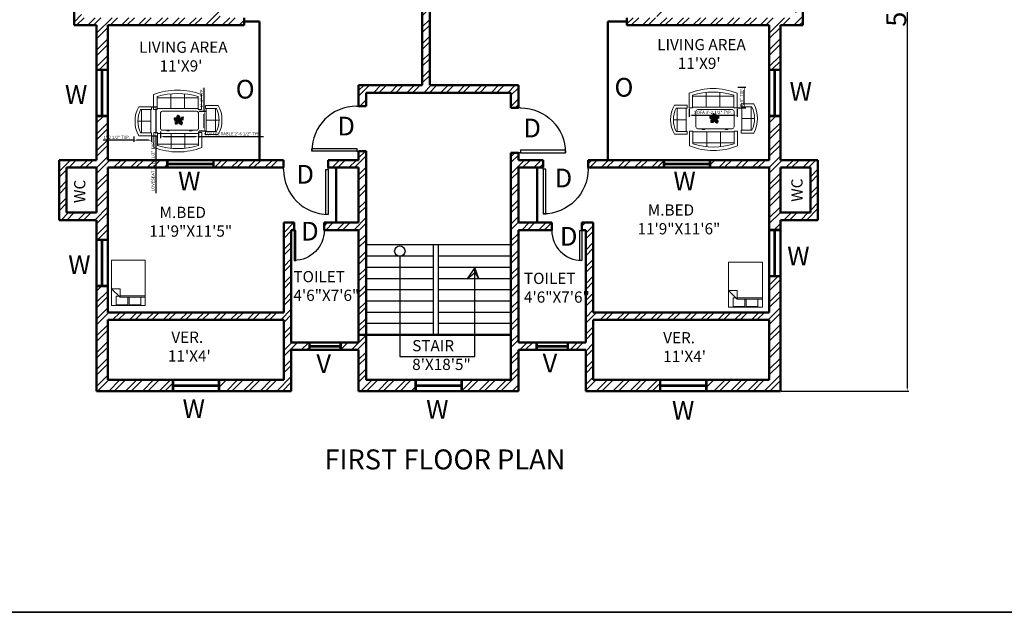
# Model space of a CAD drawing. Units: inches. Extents: x -31485 to -28799, y 18003 to 19130.
# Tile 8 of 15: x -30506 to -29717, y 18003 to 18478. Entities that reach past the tile are written whole.
import ezdxf

# ---------------------------------------------------------------- set-up
doc = ezdxf.new("R2010")
doc.units = ezdxf.units.IN
for name, color, linetype, lineweight in [('A-ANNO-DIMS', 2, 'Continuous', 18), ('A-ANNO-TEXT', 7, 'Continuous', 18), ('A-ANNO-TTLB', 7, 'Continuous', 35), ('A-AREA-IDEN', 7, 'Continuous', 18), ('A-DOOR', 3, 'Continuous', 25), ('A-FLOR-STRS', 3, 'Continuous', 25), ('A-FURN', 8, 'Continuous', 18), ('A-GLAZ', 4, 'Continuous', 25), ('A-WALL', 7, 'Continuous', 50), ('A-WALL-PATT', 8, 'Continuous', 13)]:
    doc.layers.add(name, color=color, linetype=linetype, lineweight=lineweight)
doc.styles.get("Standard").update_dxf_attribs({"font": 'arial.ttf'})
doc.dimstyles.new('ISO-25', dxfattribs={"dimtxt": 2.5, "dimasz": 2.5, "dimexe": 1.25, "dimexo": 0.625, "dimtad": 1, "dimdec": 0, "dimlunit": 3, "dimtxsty": 'Standard', "dimcen": 2.5, "dimadec": 0, "dimazin": 0, "dimtfac": 1, "dimtdec": 0, "dimtmove": 0, "dimatfit": 3, "dimfxl": 1, "dimarcsym": 0})

# ---------------------------------------------------------------- blocks, each defined once
blk = doc.blocks.new('*U8')
for p, q in [((0, 0), (0, -100)), ((750, 0), (750, -100))]:
    blk.add_line(p, q)
blk.add_lwpolyline([(0, 0), (0, 750), (43.75, 750), (43.75, 0)], close=True)
blk.add_arc((0, 0), 750, 0, 90)
blk = doc.blocks.new('Bed - Queen')
for p, q in [((0, -80.00003), (0, 0)), ((0, 0), (59.99999, 0)), ((59.99999, 0), (59.99999, -80.00003)), ((0, -14.4), (44.8, -14.4)), ((44.8, -16.8), (0, -16.8)), ((7.99999, -1.2), (28.79998, -1.2)), ((7.99999, -14.4), (7.99999, -1.2)), ((28.79998, -1.2), (28.79998, -14.4)), ((31.19999, -1.2), (51.99999, -1.2)), ((31.19999, -14.4), (31.19999, -1.2)), ((59.99999, -29.6), (44.8, -14.4)), ((44.8, -14.4), (44.8, -29.6)), ((51.99999, -16.4), (46.79936, -16.4)), ((51.99999, -1.2), (51.99999, -16.4)), ((44.8, -29.6), (59.99999, -29.6)), ((59.99999, -80.00003), (0, -80.00003))]:
    blk.add_line(p, q)
blk = doc.blocks.new('Desk - 30 x 60 in.')
for p, q in [((-26.999995, 0), (26.999995, 0)), ((-29.999995, -27), (-29.999995, -3)), ((29.999995, -3), (29.999995, -27)), ((26.999995, -30), (-26.999995, -30)), ((-20.000005, -30), (-20.000005, -31)), ((-16.000005, -31), (-16.000005, -30)), ((15.999995, -31), (15.999995, -30)), ((19.999995, -30), (19.999995, -31)), ((-20.000005, -31), (-16.000005, -31)), ((19.999995, -31), (15.999995, -31))]:
    blk.add_line(p, q)
for centre, start, end in [((-26.499995, -3.5), 98.1301, 171.8699), ((26.499995, -3.5), 8.130102, 81.8699), ((-26.499995, -26.5), 188.1301, 261.8699), ((26.499995, -26.5), 278.1301, 351.8699)]:
    blk.add_arc(centre, 3.535534, start, end)
blk = doc.blocks.new('Sofa - Roundback 7 ft.')
for p, q in [((-36.000027, -34), (-36.000027, -11.4696)), ((-35.999844, -13.3819), (35.9998, -13.3819)), ((-12.00002, -32.4421), (-12.00003, -6.5971)), ((11.99997, -32.4421), (11.99998, -6.5971)), ((35.99998, -34), (35.99998, -11.4696)), ((-36.000027, -32.4421), (35.99998, -32.4421))]:
    blk.add_line(p, q)
for points in [[(-36.000027, -34), (-42.000027, -34), (-42.000027, -8)], [(41.99998, -8), (41.99998, -34), (35.99998, -34)]]:
    blk.add_lwpolyline(points)
for centre, radius, start, end in [((0, -114.25), 114.25, 68.43141, 111.5686), ((-0.00001, -127.1968), 121.1968, 72.72033, 107.2797)]:
    blk.add_arc(centre, radius, start, end)
blk = doc.blocks.new('Sofa - Roundback Loveseat 5 ft.')
for p, q in [((-24, -33.99998), (-24, -11.46958)), ((-23.9998, -13.38178), (23.99986, -13.38178)), ((0, -32.44198), (0, -5.99998)), ((24.00004, -33.99998), (24.00004, -11.46958)), ((-24, -32.44198), (24.00004, -32.44198))]:
    blk.add_line(p, q)
for points in [[(-24, -33.99998), (-30, -33.99998), (-30, -7.99998)], [(30.00004, -7.99998), (30.00004, -33.99998), (24.00004, -33.99998)]]:
    blk.add_lwpolyline(points)
for centre, radius, start, end in [((0, -60.24998), 60.24998, 60.13715, 119.8628), ((0, -61.38438), 55.38444, 64.32083, 115.6792)]:
    blk.add_arc(centre, radius, start, end)
blk = doc.blocks.new('*U122')
for p, q in [((-1206.4492, 501.3198), (-1418.082, 465.9376)), ((-1031.621, 347.98), (-1399.667, 277.1902)), ((-800.1, 114.3), (-1333.5, 647.7)), ((-847.598, 159.2326), (-1326.0578, 135.636)), ((-1234.059, 536.7274), (-1252.4486, 737.2604)), ((-718.7946, 88.4682), (-1215.644, -147.447)), ((-1105.2302, 725.4494), (-1077.6458, 395.1732)), ((-976.4268, 666.4706), (-884.4026, 194.6402)), ((-543.9664, 76.6572), (-967.2066, -206.4512)), ((-902.8176, 713.6638), (-617.5756, 100.2538)), ((0, 0), (-800.1, 114.3)), ((-369.1382, 53.086), (-783.1836, 642.874)), ((-405.9428, 53.086), (-764.794, -241.8334)), ((-93.091, 489.5342), (-700.3796, 902.3858)), ((-129.8956, 713.6638), (-626.7704, 1032.1544)), ((-617.5756, 607.4918), (-74.7014, 347.98)), ((0, 0), (-571.5, -495.3)), ((-185.1152, 1008.5578), (-553.1612, 1185.4942)), ((-166.7002, 29.4894), (-543.9664, -206.4512)), ((-525.5514, 347.98), (-28.6766, 123.8504)), ((-221.9198, 1197.3052), (-433.5526, 1338.8594)), ((-258.7244, 1362.456), (-332.3336, 1421.4348)), ((0, 0), (-266.7, 1447.8)), ((-231.1146, 1315.2628), (-166.7002, 1421.4348)), ((-194.31, 1102.9442), (-65.4812, 1256.284)), ((-148.3106, 914.1968), (118.5418, 1220.9018)), ((-129.8956, 701.8528), (265.7602, 1185.4942)), ((-74.7014, 418.7444), (219.7608, 961.39)), ((-28.6766, 171.0436), (228.9556, 678.2816)), ((0, 0), (685.8, 228.6)), ((0, 0), (457.2, -571.5)), ((100.1268, 41.275), (284.1498, 619.2774)), ((164.5412, 41.275), (661.416, -218.2368)), ((256.5654, 88.4682), (449.7832, 666.4706)), ((284.1498, 88.4682), (781.0246, -147.447)), ((412.9786, 147.447), (587.8068, 796.2392)), ((458.978, 147.447), (891.4384, -88.4682)), ((560.197, 182.8292), (698.2206, 819.8358)), ((615.4166, 194.6402), (1185.8752, 41.275)), ((685.8, 228.6), (1219.2, 914.4)), ((689.0258, 230.0224), (790.2448, 914.1968)), ((753.4148, 312.5978), (1222.6798, 159.2326)), ((808.6344, 784.4282), (827.0494, 418.7444)), ((845.439, 418.7444), (1241.0948, 277.1902)), ((891.4384, 831.6214), (946.658, 572.1096)), ((919.0482, 501.3198), (1222.6798, 454.152)), ((983.4626, 867.0036), (1066.2666, 725.4494)), ((1029.462, 654.685), (1241.0948, 631.0884)), ((1112.2914, 760.8316), (1296.3144, 784.4282)), ((1121.4862, 925.9824), (1149.0706, 831.6214)), ((-442.7474, -383.3876), (-1086.8406, -477.7486)), ((-718.7946, -737.2604), (-1086.8406, -796.2392)), ((-617.5756, -548.5384), (-1077.6458, -560.324)), ((-783.1836, -867.029), (-1077.6458, -902.4112)), ((-875.2078, -1008.5832), (-1040.8412, -1079.3476)), ((-681.9646, -666.496), (-1022.4262, -654.685)), ((-571.5, -495.3), (-952.5, -1143)), ((-829.2084, -937.7934), (-810.7934, -1126.5408)), ((-387.5278, -324.4088), (-764.794, -324.4088)), ((-737.1842, -784.4536), (-709.5744, -1114.7298)), ((-635.9652, -607.5172), (-580.771, -1150.1374)), ((-525.5514, -465.963), (-451.9422, -1126.5408)), ((-166.7002, -147.447), (-507.1618, -253.619)), ((-433.5526, -383.3876), (-323.1134, -1020.3688)), ((-341.5284, -289.0012), (-221.9198, -831.6214)), ((-240.3094, -218.2368), (-157.5054, -595.7062)), ((-120.7008, -88.4682), (-93.091, -371.5766)), ((63.3222, -76.6826), (-37.8714, -513.1308)), ((44.9326, -64.897), (615.4166, -241.8334)), ((127.7366, -159.258), (54.1274, -654.685)), ((228.9556, -289.0012), (90.932, -914.1968)), ((357.759, -430.5554), (164.5412, -1020.3688)), ((192.151, -230.0224), (817.8292, -371.5766)), ((458.978, -572.1096), (210.5406, -1161.923)), ((311.7596, -383.3876), (937.4378, -477.7486)), ((514.1976, -772.6426), (403.7838, -1138.3264)), ((412.9786, -501.3452), (919.0482, -583.9206)), ((457.2, -571.5), (685.8, -1333.5)), ((468.1982, -572.1096), (1029.462, -737.2604)), ((486.5878, -642.8994), (983.4626, -843.4324)), ((578.612, -961.39), (495.7826, -1232.7128)), ((541.8074, -831.6214), (992.6574, -1032.1544)), ((578.612, -973.1756), (873.0488, -1138.3264)), ((624.6114, -1161.923), (587.8068, -1291.6916)), ((624.6114, -1102.9442), (781.0246, -1209.1162)), ((679.8056, -1268.095), (716.6102, -1291.6916))]:
    blk.add_line(p, q)
blk = doc.blocks.new('*D189')
at = {"layer": 'A-ANNO-DIMS', "color": 0, "lineweight": -2, "transparency": 16777216}
for p, q in [((-29895.58, 18824.12), (-29793.36, 18824.12)), ((-29794.61, 18821.62), (-29794.61, 18182.62)), ((-29895.58, 18180.12), (-29793.36, 18180.12))]:
    blk.add_line(p, q, dxfattribs=at)
at = {"layer": 'A-ANNO-DIMS', "color": 0, "transparency": 16777216}
for points in [[(-29795.03, 18821.62), (-29794.19, 18821.62), (-29794.61, 18824.12)], [(-29795.03, 18182.62), (-29794.19, 18182.62), (-29794.61, 18180.12)]]:
    blk.add_solid(points, dxfattribs=at)
at = {"layer": 'Defpoints', "color": 0, "transparency": 16777216}
for p in [(-29896.21, 18824.12), (-29896.21, 18180.12), (-29794.61, 18180.12)]:
    blk.add_point(p, dxfattribs=at)
at = {"layer": 'A-ANNO-DIMS', "color": 0, "transparency": 16777216, "insert": (-29803.41, 18502.12), "char_height": 2.5, "attachment_point": 5, "rotation": 90}
blk.add_mtext('{\\H6.4x;53\'-8"}', dxfattribs=at)
blk = doc.blocks.new('WIN-900-W9')
for p, q in [((-29982.21, 18824.12), (-29982.21, 18815.12)), ((-29981.21, 18824.12), (-29981.21, 18815.12)), ((-29981.21, 18820.12), (-29945.21, 18820.12)), ((-29981.21, 18819.62), (-29945.21, 18819.62)), ((-29981.21, 18819.12), (-29945.21, 18819.12)), ((-29945.21, 18824.12), (-29945.21, 18815.12)), ((-29944.21, 18824.12), (-29944.21, 18815.12))]:
    blk.add_line(p, q)
blk = doc.blocks.new('WIN-900-W6')
for p, q in [((-30183.21, 18720.12), (-30177.21, 18720.12)), ((-30183.21, 18719.12), (-30177.21, 18719.12)), ((-30180.71, 18683.12), (-30180.71, 18719.12)), ((-30180.21, 18683.12), (-30180.21, 18719.12)), ((-30179.71, 18683.12), (-30179.71, 18719.12)), ((-30183.21, 18683.12), (-30177.21, 18683.12)), ((-30183.21, 18682.12), (-30177.21, 18682.12))]:
    blk.add_line(p, q)
blk = doc.blocks.new('VENT-600-W6')
for p, q in [((-29884.21, 18519.12), (-29878.21, 18519.12)), ((-29884.21, 18518.12), (-29878.21, 18518.12)), ((-29881.71, 18494.12), (-29881.71, 18518.12)), ((-29881.21, 18494.12), (-29881.21, 18518.12)), ((-29880.71, 18494.12), (-29880.71, 18518.12)), ((-29884.21, 18494.12), (-29878.21, 18494.12)), ((-29884.21, 18493.12), (-29878.21, 18493.12))]:
    blk.add_line(p, q)
blk = doc.blocks.new('*D224')
at = {"layer": 'A-ANNO-DIMS', "color": 0, "lineweight": -2, "transparency": 16777216}
for p, q in [((-30399.59, 18407.94), (-30395.47, 18407.94)), ((-30396.72, 18405.44), (-30396.72, 18387.1)), ((-30399.59, 18384.6), (-30395.47, 18384.6)), ((-30396.72, 18384.6), (-30396.72, 18338.55))]:
    blk.add_line(p, q, dxfattribs=at)
at = {"layer": 'A-ANNO-DIMS', "color": 0, "transparency": 16777216}
for points in [[(-30397.13, 18405.44), (-30396.3, 18405.44), (-30396.72, 18407.94)], [(-30397.13, 18387.1), (-30396.3, 18387.1), (-30396.72, 18384.6)]]:
    blk.add_solid(points, dxfattribs=at)
at = {"layer": 'Defpoints', "color": 0, "transparency": 16777216}
for p in [(-30400.22, 18407.94), (-30400.22, 18384.6), (-30396.72, 18384.6)]:
    blk.add_point(p, dxfattribs=at)
at = {"layer": 'A-ANNO-DIMS', "color": 0, "transparency": 16777216, "insert": (-30398.63, 18360.33), "char_height": 2.5, "attachment_point": 5, "rotation": 90}
blk.add_mtext('LOVESEAT 1\'-11 1/2" TYP.', dxfattribs=at)
blk = doc.blocks.new('*D225')
at = {"layer": 'A-ANNO-DIMS', "color": 0, "lineweight": -2, "transparency": 16777216}
for p, q in [((-30414.48, 18381.1), (-30439.06, 18381.1)), ((-30414.48, 18383.98), (-30414.48, 18379.85)), ((-30402.72, 18381.1), (-30411.98, 18381.1)), ((-30400.22, 18383.98), (-30400.22, 18379.85))]:
    blk.add_line(p, q, dxfattribs=at)
at = {"layer": 'A-ANNO-DIMS', "color": 0, "transparency": 16777216}
for points in [[(-30411.98, 18381.52), (-30411.98, 18380.69), (-30414.48, 18381.1)], [(-30402.72, 18381.52), (-30402.72, 18380.69), (-30400.22, 18381.1)]]:
    blk.add_solid(points, dxfattribs=at)
at = {"layer": 'Defpoints', "color": 0, "transparency": 16777216}
for p in [(-30414.48, 18384.6), (-30414.48, 18381.1), (-30400.22, 18384.6)]:
    blk.add_point(p, dxfattribs=at)
at = {"layer": 'A-ANNO-DIMS', "color": 0, "transparency": 16777216, "insert": (-30428.02, 18383.02), "char_height": 2.5, "attachment_point": 5}
blk.add_mtext('1\'-2 1/2" TYP.', dxfattribs=at)
blk = doc.blocks.new('*D230')
at = {"layer": 'A-ANNO-DIMS', "color": 0, "lineweight": -2, "transparency": 16777216}
for p, q in [((-29969.34, 18406.26), (-29969.34, 18399.87)), ((-29966.84, 18401.12), (-29933.43, 18401.12)), ((-29930.93, 18406.26), (-29930.93, 18399.87))]:
    blk.add_line(p, q, dxfattribs=at)
at = {"layer": 'A-ANNO-DIMS', "color": 0, "transparency": 16777216}
for points in [[(-29966.84, 18401.54), (-29966.84, 18400.71), (-29969.34, 18401.12)], [(-29933.43, 18401.54), (-29933.43, 18400.71), (-29930.93, 18401.12)]]:
    blk.add_solid(points, dxfattribs=at)
at = {"layer": 'Defpoints', "color": 0, "transparency": 16777216}
for p in [(-29969.34, 18406.88), (-29930.93, 18406.88), (-29930.93, 18401.12)]:
    blk.add_point(p, dxfattribs=at)
at = {"layer": 'A-ANNO-DIMS', "color": 0, "transparency": 16777216, "insert": (-29950.13, 18403.04), "char_height": 2.5, "attachment_point": 5}
blk.add_mtext('SOFA 3\'-2 1/2" TYP.', dxfattribs=at)
blk = doc.blocks.new('*D231')
at = {"layer": 'A-ANNO-DIMS', "color": 0, "lineweight": -2, "transparency": 16777216}
for p, q in [((-29930.3, 18423.65), (-29923.92, 18423.65)), ((-29925.17, 18409.38), (-29925.17, 18421.15)), ((-29930.3, 18406.88), (-29923.92, 18406.88))]:
    blk.add_line(p, q, dxfattribs=at)
at = {"layer": 'A-ANNO-DIMS', "color": 0, "transparency": 16777216}
for points in [[(-29925.59, 18421.15), (-29924.75, 18421.15), (-29925.17, 18423.65)], [(-29925.59, 18409.38), (-29924.75, 18409.38), (-29925.17, 18406.88)]]:
    blk.add_solid(points, dxfattribs=at)
at = {"layer": 'Defpoints', "color": 0, "transparency": 16777216}
for p in [(-29930.93, 18423.65), (-29925.17, 18423.65), (-29930.93, 18406.88)]:
    blk.add_point(p, dxfattribs=at)
at = {"layer": 'A-ANNO-DIMS', "color": 0, "transparency": 16777216, "insert": (-29927.07, 18415.27), "char_height": 2.5, "attachment_point": 5, "rotation": 90}
blk.add_mtext('1\'-5" TYP.', dxfattribs=at)
blk = doc.blocks.new('*D240')
at = {"layer": 'A-ANNO-DIMS', "color": 0, "lineweight": -2, "transparency": 16777216}
for p, q in [((-30393.09, 18387.93), (-30393.09, 18382.72)), ((-30362.51, 18387.93), (-30362.51, 18382.72)), ((-30390.59, 18383.97), (-30365.01, 18383.97)), ((-30362.51, 18383.97), (-30310.56, 18383.97))]:
    blk.add_line(p, q, dxfattribs=at)
at = {"layer": 'A-ANNO-DIMS', "color": 0, "transparency": 16777216}
for points in [[(-30390.59, 18384.39), (-30390.59, 18383.55), (-30393.09, 18383.97)], [(-30365.01, 18384.39), (-30365.01, 18383.55), (-30362.51, 18383.97)]]:
    blk.add_solid(points, dxfattribs=at)
at = {"layer": 'Defpoints', "color": 0, "transparency": 16777216}
for p in [(-30393.09, 18388.56), (-30362.51, 18388.56), (-30362.51, 18383.97)]:
    blk.add_point(p, dxfattribs=at)
at = {"layer": 'A-ANNO-DIMS', "color": 0, "transparency": 16777216, "insert": (-30335.29, 18385.89), "char_height": 2.5, "attachment_point": 5}
blk.add_mtext('COFFEE TABLE 2\'-6 1/2" TYP.', dxfattribs=at)
blk = doc.blocks.new('*D241')
at = {"layer": 'A-ANNO-DIMS', "color": 0, "lineweight": -2, "transparency": 16777216}
for p, q in [((-30357.93, 18404.36), (-30357.93, 18423.11)), ((-30361.89, 18404.36), (-30356.68, 18404.36)), ((-30357.93, 18391.06), (-30357.93, 18401.86)), ((-30361.89, 18388.56), (-30356.68, 18388.56))]:
    blk.add_line(p, q, dxfattribs=at)
at = {"layer": 'A-ANNO-DIMS', "color": 0, "transparency": 16777216}
for points in [[(-30358.34, 18401.86), (-30357.51, 18401.86), (-30357.93, 18404.36)], [(-30358.34, 18391.06), (-30357.51, 18391.06), (-30357.93, 18388.56)]]:
    blk.add_solid(points, dxfattribs=at)
at = {"layer": 'Defpoints', "color": 0, "transparency": 16777216}
for p in [(-30362.51, 18404.36), (-30357.93, 18404.36), (-30362.51, 18388.56)]:
    blk.add_point(p, dxfattribs=at)
at = {"layer": 'A-ANNO-DIMS', "color": 0, "transparency": 16777216, "insert": (-30359.81, 18414.98), "char_height": 2.5, "attachment_point": 5, "rotation": 90}
blk.add_mtext('1\'-4" TYP.', dxfattribs=at)

msp = doc.modelspace()

# ---------------------------------------------------------------- hatches: boundary and pattern name
at = {"layer": 'A-WALL-PATT'}
h = msp.add_hatch(dxfattribs=at)
h.set_pattern_fill('ANSI32', color=256)
h.paths.add_polyline_path([(-30435.21, 18779.12), (-30435.21, 18815.12), (-30406.21, 18815.12), (-30406.21, 18824.12), (-30444.21, 18824.12), (-30444.21, 18779.12), (-30474.21, 18779.12), (-30474.21, 18731.12), (-30444.21, 18731.12), (-30444.21, 18704.18), (-30435.21, 18704.18), (-30435.21, 18773.12), (-30369.28, 18773.12), (-30369.28, 18779.12)])
h.paths.add_polyline_path([(-30444.21, 18773.12), (-30444.21, 18737.12), (-30468.21, 18737.12), (-30468.21, 18773.12)], flags=16)
h.paths.add_polyline_path([(-30333.21, 18824.12), (-30368.21, 18824.12), (-30368.21, 18815.12), (-30339.21, 18815.12), (-30339.21, 18779.12), (-30345.28, 18779.12), (-30345.28, 18773.12), (-30312.21, 18773.12), (-30312.21, 18629.12), (-30315.41, 18629.12), (-30315.41, 18626.12), (-30315.41, 18623.12), (-30299.19, 18623.12), (-30299.19, 18629.12), (-30306.21, 18629.12), (-30306.21, 18773.12), (-30274.83, 18773.12), (-30274.83, 18779.12), (-30279.21, 18779.12), (-30279.21, 18815.12), (-30250.21, 18815.12), (-30250.21, 18824.12), (-30285.21, 18824.12), (-30285.21, 18779.12), (-30333.21, 18779.12)])
h.paths.add_polyline_path([(-30177.21, 18779.12), (-30177.21, 18815.12), (-30148.21, 18815.12), (-30148.21, 18824.12), (-30212.21, 18824.12), (-30212.21, 18815.12), (-30183.21, 18815.12), (-30183.21, 18779.12), (-30250.83, 18779.12), (-30250.83, 18776.12), (-30250.83, 18773.12), (-30183.21, 18773.12), (-30183.21, 18720.12), (-30177.21, 18720.12), (-30177.21, 18773.12), (-30110.84, 18773.12), (-30110.84, 18779.12)])
h.paths.add_polyline_path([(-30015.86, 18779.12), (-30021.21, 18779.12), (-30021.21, 18815.12), (-29982.21, 18815.12), (-29982.21, 18824.12), (-30027.21, 18824.12), (-30027.21, 18779.12), (-30075.21, 18779.12), (-30075.21, 18824.12), (-30110.21, 18824.12), (-30110.21, 18815.12), (-30081.21, 18815.12), (-30081.21, 18779.12), (-30086.84, 18779.12), (-30086.84, 18776.12), (-30086.84, 18773.12), (-30054.21, 18773.12), (-30054.21, 18629.12), (-30058.98, 18629.12), (-30058.98, 18623.12), (-30045.32, 18623.12), (-30045.32, 18629.12), (-30048.21, 18629.12), (-30048.21, 18773.12), (-30015.86, 18773.12)])
h.paths.add_polyline_path([(-29866.21, 18779.12), (-29896.21, 18779.12), (-29896.21, 18824.12), (-29944.21, 18824.12), (-29944.21, 18815.12), (-29905.21, 18815.12), (-29905.21, 18779.12), (-29991.86, 18779.12), (-29991.86, 18776.12), (-29991.86, 18773.12), (-29905.21, 18773.12), (-29905.21, 18720.12), (-29896.21, 18720.12), (-29896.21, 18731.12), (-29866.21, 18731.12)])
h.paths.add_polyline_path([(-29896.21, 18773.12), (-29872.21, 18773.12), (-29872.21, 18737.12), (-29896.21, 18737.12)], flags=16)
h.paths.add_polyline_path([(-29896.21, 18682.12), (-29905.21, 18682.12), (-29905.21, 18629.12), (-30009.32, 18629.12), (-30009.32, 18626.12), (-30009.32, 18623.12), (-29995.21, 18623.12), (-29995.21, 18573.22), (-29989.21, 18573.22), (-29989.21, 18623.12), (-29905.21, 18623.12), (-29905.21, 18594.12), (-29896.21, 18594.12)])
h.paths.add_polyline_path([(-30094.98, 18629.12), (-30177.21, 18629.12), (-30177.21, 18682.12), (-30183.21, 18682.12), (-30183.21, 18629.12), (-30263.19, 18629.12), (-30263.19, 18626.12), (-30263.19, 18623.12), (-30183.21, 18623.12), (-30183.21, 18425.12), (-30234.21, 18425.12), (-30234.21, 18408.38), (-30228.21, 18408.38), (-30228.21, 18419.12), (-30112.21, 18419.12), (-30112.21, 18406.94), (-30106.21, 18406.94), (-30106.21, 18425.12), (-30177.21, 18425.12), (-30177.21, 18623.12), (-30094.98, 18623.12)])
h.paths.add_polyline_path([(-29896.21, 18568.12), (-29905.21, 18568.12), (-29905.21, 18539.12), (-29989.21, 18539.12), (-29989.21, 18549.22), (-29992.21, 18549.22), (-29995.21, 18549.22), (-29995.21, 18519.45), (-29989.21, 18519.45), (-29989.21, 18533.12), (-29884.21, 18533.12), (-29884.21, 18519.12), (-29878.21, 18519.12), (-29878.21, 18539.12), (-29896.21, 18539.12)])
h.paths.add_polyline_path([(-29878.21, 18493.12), (-29884.21, 18493.12), (-29884.21, 18479.12), (-29989.21, 18479.12), (-29989.21, 18495.45), (-29992.21, 18495.45), (-29995.21, 18495.45), (-29995.21, 18479.12), (-30019.21, 18479.12), (-30019.21, 18473.12), (-29905.21, 18473.12), (-29905.21, 18438.12), (-29896.21, 18438.12), (-29896.21, 18473.12), (-29878.21, 18473.12)])
h.paths.add_polyline_path([(-29896.21, 18400.12), (-29905.21, 18400.12), (-29905.21, 18365.12), (-29952.21, 18365.12), (-29952.21, 18359.12), (-29905.21, 18359.12), (-29905.21, 18309.79), (-29896.21, 18309.79), (-29896.21, 18317.12), (-29866.21, 18317.12), (-29866.21, 18365.12), (-29896.21, 18365.12)])
h.paths.add_polyline_path([(-29896.21, 18359.12), (-29872.21, 18359.12), (-29872.21, 18323.12), (-29896.21, 18323.12)], flags=16)
h.paths.add_polyline_path([(-29990.21, 18365.12), (-30043.21, 18365.12), (-30050.35, 18365.12), (-30050.35, 18359.12), (-29990.21, 18359.12)])
h.paths.add_polyline_path([(-29896.21, 18271.79), (-29905.21, 18271.79), (-29905.21, 18243.12), (-30046.21, 18243.12), (-30046.21, 18315.12), (-30055.46, 18315.12), (-30055.46, 18309.12), (-30052.21, 18309.12), (-30052.21, 18219.12), (-30066.21, 18219.12), (-30066.21, 18213.12), (-30052.21, 18213.12), (-30052.21, 18180.12), (-29993.21, 18180.12), (-29993.21, 18189.12), (-30046.21, 18189.12), (-30046.21, 18237.12), (-29905.21, 18237.12), (-29905.21, 18189.12), (-29955.21, 18189.12), (-29955.21, 18180.12), (-29896.21, 18180.12)])
h.paths.add_polyline_path([(-30092.21, 18219.12), (-30106.21, 18219.12), (-30106.21, 18309.12), (-30079.46, 18309.12), (-30079.46, 18315.12), (-30106.21, 18315.12), (-30106.21, 18359.12), (-30086.35, 18359.12), (-30086.35, 18365.12), (-30106.21, 18365.12), (-30106.21, 18370.94), (-30112.21, 18370.94), (-30112.21, 18189.12), (-30151.21, 18189.12), (-30151.21, 18180.12), (-30106.21, 18180.12), (-30106.21, 18213.12), (-30092.21, 18213.12)])
h.paths.add_polyline_path([(-30189.21, 18189.12), (-30228.21, 18189.12), (-30228.21, 18225.12), (-30234.21, 18225.12), (-30234.21, 18219.12), (-30248.21, 18219.12), (-30248.21, 18213.12), (-30234.21, 18213.12), (-30234.21, 18180.12), (-30189.21, 18180.12)])
h.paths.add_polyline_path([(-30288.21, 18213.12), (-30274.21, 18213.12), (-30274.21, 18219.12), (-30288.21, 18219.12), (-30288.21, 18309.12), (-30285.87, 18309.12), (-30285.87, 18315.12), (-30294.21, 18315.12), (-30294.21, 18243.12), (-30435.21, 18243.12), (-30435.21, 18263.9), (-30444.21, 18263.9), (-30444.21, 18180.12), (-30383.71, 18180.12), (-30383.71, 18189.12), (-30435.21, 18189.12), (-30435.21, 18237.12), (-30294.21, 18237.12), (-30294.21, 18189.12), (-30345.71, 18189.12), (-30345.71, 18180.12), (-30288.21, 18180.12)])
h.paths.add_polyline_path([(-30435.21, 18359.12), (-30388.21, 18359.12), (-30388.21, 18365.12), (-30435.21, 18365.12), (-30435.21, 18400.12), (-30444.21, 18400.12), (-30444.21, 18365.12), (-30474.21, 18365.12), (-30474.21, 18317.12), (-30444.21, 18317.12), (-30444.21, 18301.9), (-30435.21, 18301.9)])
h.paths.add_polyline_path([(-30444.21, 18323.12), (-30468.21, 18323.12), (-30468.21, 18359.12), (-30444.21, 18359.12)], flags=16)
h.paths.add_polyline_path([(-30294.54, 18365.12), (-30297.21, 18365.12), (-30350.21, 18365.12), (-30350.21, 18359.12), (-30294.54, 18359.12)])
h.paths.add_polyline_path([(-30228.21, 18372.38), (-30234.21, 18372.38), (-30234.21, 18365.12), (-30258.54, 18365.12), (-30258.54, 18359.12), (-30234.21, 18359.12), (-30234.21, 18315.12), (-30261.87, 18315.12), (-30261.87, 18309.12), (-30234.21, 18309.12), (-30234.21, 18225.12), (-30228.21, 18225.12)])
h.paths.add_polyline_path([(-30375.49, 18525.25), (-30375.54, 18525.25), (-30375.54, 18526.65), (-30351.51, 18526.65), (-30351.51, 18525.25), (-30375.49, 18525.25, 0.400923), (-30351.21, 18502.63), (-30351.21, 18502.64), (-30345.21, 18502.64), (-30345.21, 18479.12), (-30325.98, 18479.12), (-30325.98, 18473.12), (-30435.21, 18473.12), (-30435.21, 18437.12), (-30439.21, 18437.12), (-30439.21, 18401.12), (-30440.21, 18401.12), (-30440.21, 18437.12), (-30444.21, 18437.12), (-30444.21, 18473.12), (-30462.21, 18473.12), (-30462.21, 18494.12), (-30456.21, 18494.12), (-30456.21, 18479.12), (-30351.21, 18479.12), (-30351.21, 18502.63), (-30351.51, 18502.63, -0.39722)])
h.paths.add_polyline_path([(-30345.21, 18556.53), (-30351.21, 18556.53), (-30351.21, 18539.12), (-30435.21, 18539.12), (-30435.21, 18568.12), (-30444.21, 18568.12), (-30444.21, 18539.12), (-30462.21, 18539.12), (-30462.21, 18519.12), (-30456.21, 18519.12), (-30456.21, 18533.12), (-30351.21, 18533.12), (-30351.21, 18526.64), (-30345.21, 18526.64)])
h.paths.add_polyline_path([(-30344.41, 18629.12), (-30435.21, 18629.12), (-30435.21, 18666.18), (-30444.21, 18666.18), (-30444.21, 18594.12), (-30435.21, 18594.12), (-30435.21, 18623.12), (-30351.21, 18623.12), (-30351.21, 18580.56), (-30347.87, 18580.56), (-30345.21, 18580.53), (-30345.21, 18623.12)])

# ---------------------------------------------------------------- linework, layer by layer
at = {"layer": 'A-ANNO-TTLB'}
msp.add_lwpolyline([(-31485.1, 19129.94), (-28798.64, 19129.94), (-28798.64, 18002.86), (-31485.1, 18002.86)], close=True, dxfattribs=at)
at = {"layer": 'A-FLOR-STRS'}
for p, q in [((-30112.21, 18297.12), (-30228.21, 18297.12)), ((-30174.21, 18225.12), (-30174.21, 18297.12)), ((-30170.21, 18225.12), (-30170.21, 18297.12)), ((-30174.21, 18288.12), (-30228.21, 18288.12)), ((-30201.21, 18288.12), (-30201.21, 18207.7)), ((-30112.21, 18288.12), (-30170.21, 18288.12)), ((-30174.21, 18279.12), (-30228.21, 18279.12)), ((-30112.21, 18279.12), (-30170.21, 18279.12)), ((-30141.21, 18279.12), (-30147.29, 18270.12)), ((-30147.29, 18270.12), (-30141.21, 18275.01)), ((-30141.21, 18207.7), (-30141.21, 18279.12)), ((-30138.01, 18270.12), (-30141.21, 18279.12)), ((-30141.21, 18275.01), (-30138.01, 18270.12)), ((-30174.21, 18270.12), (-30228.21, 18270.12)), ((-30112.21, 18270.12), (-30170.21, 18270.12)), ((-30174.21, 18261.12), (-30228.21, 18261.12)), ((-30112.21, 18261.12), (-30170.21, 18261.12)), ((-30174.21, 18252.12), (-30228.21, 18252.12)), ((-30112.21, 18252.12), (-30170.21, 18252.12)), ((-30174.21, 18243.12), (-30228.21, 18243.12)), ((-30112.21, 18243.12), (-30170.21, 18243.12)), ((-30174.21, 18234.12), (-30228.21, 18234.12)), ((-30112.21, 18234.12), (-30170.21, 18234.12)), ((-30201.21, 18207.7), (-30141.21, 18207.7))]:
    msp.add_line(p, q, dxfattribs=at)
msp.add_circle((-30201.21, 18292.29), 4.17, dxfattribs=at)
at = {"layer": 'A-WALL'}
for p, q in [((-30183.21, 18425.12), (-30183.21, 18623.12)), ((-30177.21, 18425.12), (-30177.21, 18623.12)), ((-30462.21, 18473.12), (-30462.21, 18539.12)), ((-29878.21, 18539.12), (-29878.21, 18473.12)), ((-30462.21, 18473.12), (-30444.21, 18473.12)), ((-30444.21, 18365.12), (-30444.21, 18473.12)), ((-30435.21, 18473.12), (-30325.98, 18473.12)), ((-30435.21, 18365.12), (-30435.21, 18473.12)), ((-30325.98, 18479.12), (-30325.98, 18473.12)), ((-30313.56, 18476.12), (-30325.98, 18476.12)), ((-30313.56, 18365.12), (-30313.56, 18476.12)), ((-30034.63, 18365.12), (-30034.63, 18476.12)), ((-30034.63, 18476.12), (-30019.21, 18476.12)), ((-30019.21, 18479.12), (-30019.21, 18473.12)), ((-30019.21, 18473.12), (-29905.21, 18473.12)), ((-29905.21, 18473.12), (-29905.21, 18365.12)), ((-29896.21, 18473.12), (-29896.21, 18365.12)), ((-29896.21, 18473.12), (-29878.21, 18473.12)), ((-30234.21, 18425.12), (-30183.21, 18425.12)), ((-30234.21, 18408.38), (-30234.21, 18425.12)), ((-30177.21, 18425.12), (-30106.21, 18425.12)), ((-30106.21, 18425.12), (-30106.21, 18406.94)), ((-30228.21, 18419.12), (-30112.21, 18419.12)), ((-30228.21, 18408.38), (-30228.21, 18419.12)), ((-30112.21, 18419.12), (-30112.21, 18406.94)), ((-30234.21, 18408.38), (-30228.21, 18408.38)), ((-30112.21, 18406.94), (-30106.21, 18406.94)), ((-30234.21, 18365.12), (-30234.21, 18372.38)), ((-30234.21, 18372.38), (-30228.21, 18372.38)), ((-30228.21, 18189.12), (-30228.21, 18372.38)), ((-30112.21, 18370.94), (-30106.21, 18370.94)), ((-30112.21, 18370.94), (-30112.21, 18189.12)), ((-30106.21, 18370.94), (-30106.21, 18365.12)), ((-30474.21, 18365.12), (-30444.21, 18365.12)), ((-30474.21, 18317.12), (-30474.21, 18365.12)), ((-30435.21, 18365.12), (-30297.21, 18365.12)), ((-30297.21, 18365.12), (-30294.54, 18365.12)), ((-30294.54, 18365.12), (-30294.54, 18359.12)), ((-30258.54, 18365.12), (-30258.54, 18359.12)), ((-30258.54, 18365.12), (-30234.21, 18365.12)), ((-30106.21, 18365.12), (-30086.35, 18365.12)), ((-30086.35, 18365.12), (-30086.35, 18359.12)), ((-30050.35, 18365.12), (-30050.35, 18359.12)), ((-30050.35, 18365.12), (-30043.21, 18365.12)), ((-30043.21, 18365.12), (-29905.21, 18365.12)), ((-29896.21, 18365.12), (-29866.21, 18365.12)), ((-29866.21, 18365.12), (-29866.21, 18317.12)), ((-30468.21, 18359.12), (-30444.21, 18359.12)), ((-30468.21, 18323.12), (-30468.21, 18359.12)), ((-30444.21, 18323.12), (-30444.21, 18359.12)), ((-30435.21, 18243.12), (-30435.21, 18359.12)), ((-30435.21, 18359.12), (-30294.54, 18359.12)), ((-30258.54, 18359.12), (-30234.21, 18359.12)), ((-30252.12, 18359.12), (-30252.12, 18315.12)), ((-30234.21, 18315.12), (-30234.21, 18359.12)), ((-30106.21, 18359.12), (-30086.35, 18359.12)), ((-30106.21, 18359.12), (-30106.21, 18315.12)), ((-30091.15, 18359.12), (-30091.15, 18315.12)), ((-30050.35, 18359.12), (-29905.21, 18359.12)), ((-29905.21, 18359.12), (-29905.21, 18243.12)), ((-29896.21, 18359.12), (-29896.21, 18323.12)), ((-29896.21, 18359.12), (-29872.21, 18359.12)), ((-29872.21, 18359.12), (-29872.21, 18323.12)), ((-30468.21, 18323.12), (-30444.21, 18323.12)), ((-29896.21, 18323.12), (-29872.21, 18323.12)), ((-30474.21, 18317.12), (-30444.21, 18317.12)), ((-30444.21, 18180.12), (-30444.21, 18317.12)), ((-30294.21, 18243.12), (-30294.21, 18315.12)), ((-30285.87, 18315.12), (-30294.21, 18315.12)), ((-30285.87, 18309.12), (-30285.87, 18315.12)), ((-30234.21, 18315.12), (-30261.87, 18315.12)), ((-30261.87, 18309.12), (-30261.87, 18315.12)), ((-30079.46, 18315.12), (-30106.21, 18315.12)), ((-30079.46, 18309.12), (-30079.46, 18315.12)), ((-30046.21, 18315.12), (-30055.46, 18315.12)), ((-30055.46, 18309.12), (-30055.46, 18315.12)), ((-30046.21, 18315.12), (-30046.21, 18243.12)), ((-29896.21, 18317.12), (-29866.21, 18317.12)), ((-29896.21, 18317.12), (-29896.21, 18180.12)), ((-30288.21, 18219.12), (-30288.21, 18309.12)), ((-30285.87, 18309.12), (-30288.21, 18309.12)), ((-30234.21, 18309.12), (-30261.87, 18309.12)), ((-30234.21, 18219.12), (-30234.21, 18309.12)), ((-30106.21, 18309.12), (-30106.21, 18219.12)), ((-30079.46, 18309.12), (-30106.21, 18309.12)), ((-30052.21, 18309.12), (-30055.46, 18309.12)), ((-30052.21, 18309.12), (-30052.21, 18219.12)), ((-30294.21, 18243.12), (-30435.21, 18243.12)), ((-29905.21, 18243.12), (-30046.21, 18243.12)), ((-30435.21, 18189.12), (-30435.21, 18237.12)), ((-30294.21, 18237.12), (-30435.21, 18237.12)), ((-30294.21, 18189.12), (-30294.21, 18237.12)), ((-29905.21, 18237.12), (-30046.21, 18237.12)), ((-30046.21, 18237.12), (-30046.21, 18189.12)), ((-29905.21, 18237.12), (-29905.21, 18189.12)), ((-30112.21, 18225.12), (-30234.21, 18225.12)), ((-30234.21, 18219.12), (-30288.21, 18219.12)), ((-30288.21, 18180.12), (-30288.21, 18213.12)), ((-30234.21, 18213.12), (-30288.21, 18213.12)), ((-30234.21, 18180.12), (-30234.21, 18213.12)), ((-30052.21, 18219.12), (-30106.21, 18219.12)), ((-30052.21, 18213.12), (-30106.21, 18213.12)), ((-30106.21, 18213.12), (-30106.21, 18180.12)), ((-30052.21, 18213.12), (-30052.21, 18180.12)), ((-30294.21, 18189.12), (-30435.21, 18189.12)), ((-30112.21, 18189.12), (-30228.21, 18189.12)), ((-29905.21, 18189.12), (-30046.21, 18189.12)), ((-30288.21, 18180.12), (-30444.21, 18180.12)), ((-30106.21, 18180.12), (-30234.21, 18180.12)), ((-29896.21, 18180.12), (-30052.21, 18180.12))]:
    msp.add_line(p, q, dxfattribs=at)

# ---------------------------------------------------------------- block references
at = {"layer": 'A-DOOR'}
for p, xscale, yscale, zscale, rotation in [((-30235.8, 18372.4), 0.0479138447310686, 0.0479138447310686, 0.0479138447310686, 90.00000000000003), ((-30104.41, 18370.94), -0.0480000229587316, 0.0480000229587316, 0.0480000229587316, 270), ((-30258.54, 18357.57), 0.0478432721548592, 0.0478432721548592, 0.0478432721548592, 180), ((-30086.35, 18358), -0.048000000000011, 0.048000000000011, 0.048000000000011, 180), ((-30285.85, 18308.8), -0.0320000000000009, 0.0320000000000009, 0.0320000000000009, 180), ((-30055.46, 18308.78), 0.0319722917760897, 0.0319722917760897, 0.0319722917760897, 180)]:
    msp.add_blockref('*U8', p, dxfattribs=dict(at, xscale=xscale, yscale=yscale, zscale=zscale, rotation=rotation))
at = {"layer": 'A-FURN'}
for name, p, xscale, yscale, zscale in [('Sofa - Roundback 7 ft.', (-30379.33, 18421.24), 0.4572254050602915, 0.4572254050602915, 0.4572254050602915), ('Sofa - Roundback 7 ft.', (-29950.13, 18422.43), 0.4572254050602915, 0.4572254050602915, 0.4572254050602915), ('Desk - 30 x 60 in.', (-30377.8, 18404.36), 0.509642021905153, 0.509642021905153, 0.509642021905153), ('*U122', (-30378.24, 18397.13), 0.0029334549167862, 0.0029334549167862, 0.0029334549167862), ('Desk - 30 x 60 in.', (-29948.61, 18405.55), 0.509642021905153, 0.509642021905153, 0.509642021905153), ('*U122', (-29948.96, 18398.37), 0.0029334549167862, 0.0029334549167862, 0.0029334549167862)]:
    msp.add_blockref(name, p, dxfattribs=dict(at, xscale=xscale, yscale=yscale, zscale=zscale))
for name, p, xscale, yscale, zscale, rotation in [('Sofa - Roundback Loveseat 5 ft.', (-30343.73, 18397.26), 0.3890039432430373, 0.3890039432430373, 0.3890039432430373, 270), ('Sofa - Roundback Loveseat 5 ft.', (-29984.25, 18397.46), -0.3890039432430373, 0.3890039432430373, 0.3890039432430373, 90), ('Sofa - Roundback Loveseat 5 ft.', (-29914.53, 18398.45), 0.3890039432430373, 0.3890039432430373, 0.3890039432430373, 270), ('Sofa - Roundback Loveseat 5 ft.', (-30413.44, 18396.27), -0.3890039432430373, 0.3890039432430373, 0.3890039432430373, 90), ('Sofa - Roundback 7 ft.', (-30379.03, 18371.65), -0.4572254050602915, 0.4572254050602915, 0.4572254050602915, 180), ('Sofa - Roundback 7 ft.', (-29949.83, 18372.84), -0.4572254050602915, 0.4572254050602915, 0.4572254050602915, 180), ('Bed - Queen', (-30405.19, 18248.72), 0.4514551267732207, 0.4514551267732207, 0.4514551267732207, 180), ('Bed - Queen', (-29910.69, 18247.32), 0.4514551267732207, 0.4514551267732207, 0.4514551267732207, 180)]:
    msp.add_blockref(name, p, dxfattribs=dict(at, xscale=xscale, yscale=yscale, zscale=zscale, rotation=rotation))
at = {"layer": 'A-GLAZ'}
for name, p, rotation in [('WIN-900-W9', (-11620.09, 48382.32), 90.00000000002325), ('WIN-900-W9', (-11081.09, 48382.32), 89.99999999999207), ('WIN-900-W6', (-49070.32, -11818.09), 270.0000000000192), ('WIN-900-W6', (-48672.32, -11818.09), 270.0000000000124), ('WIN-900-W9', (-11081.09, 48254), 89.9999999999847), ('WIN-900-W9', (-11620.09, 48246.11), 89.9999999999847), ('VENT-600-W6', (-48767.32, -11665.09), 270.0000000000538), ('VENT-600-W6', (-48585.32, -11665.09), 270.0000000000082)]:
    msp.add_blockref(name, p, dxfattribs=dict(at, rotation=rotation))
for p in [(-401.5, -635), (-207, -635), (-11, -635)]:
    msp.add_blockref('WIN-900-W9', p, dxfattribs=at)

# ---------------------------------------------------------------- texts
at = {"layer": 'A-ANNO-TEXT', "attachment_point": 1}
for s, width, insert, char_height in [('{W}', 1155.9407, (-30469.56, 18425.17), 15), ('{O}', 1155.9407, (-30332.74, 18429.44), 15), ('{O}', 1155.9407, (-30029.21, 18430.94), 15), ('{W}', 1155.9407, (-29888.91, 18427.67), 15), ('{D}', 1155.9407, (-30251.25, 18399.87), 15), ('{D}', 1155.9407, (-30102.19, 18398.31), 15), ('{W}', 1155.9407, (-30378.94, 18355.86), 15), ('{D}', 1155.9407, (-30284.1, 18361.25), 15), ('{D}', 1155.9407, (-30077.14, 18358.27), 15), ('{W}', 1155.9407, (-29981.99, 18355.94), 15), ('{D}', 1155.9407, (-30280.31, 18315.67), 15), ('{D}', 1155.9407, (-30072.93, 18311.55), 15), ('{W}', 1155.9407, (-29890.78, 18295.91), 15), ('{W}', 1155.9407, (-30466.99, 18288.97), 15), ('{V}', 1155.9407, (-30268.12, 18209.62), 15), ('{V}', 1155.9407, (-30086.8, 18210.08), 15), ('{W}', 1155.9407, (-30375.34, 18173.49), 15), ('{W}', 1155.9407, (-30180.12, 18173), 15), ('{W}', 1155.9407, (-29983.16, 18172.14), 15), ('{FIRST FLOOR PLAN}', 991.984, (-30261.61, 18133.33), 16)]:
    msp.add_mtext_dynamic_manual_height_columns(s, width=width, gutter_width=12.5, heights=[0], dxfattribs=dict(at, insert=insert, char_height=char_height))
at = {"layer": 'A-AREA-IDEN', "char_height": 9, "attachment_point": 1}
for s, heights, insert in [("{LIVING AREA\\P      11'X9'}", [0], (-30410.21, 18460.09)), ("{ LIVING AREA\\P       11'X9'}", [0], (-29997.69, 18462.15)), ('{   M.BED\\P11\'9"X11\'5"}', [0], (-30401.98, 18327.77)), ('{   M.BED\\P11\'9"X11\'6"}', [0], (-30010.75, 18329.66)), ('{  TOILET\\P  4\'6"X7\'6"}', [0], (-30291.99, 18276.28)), ('{   TOILET\\P   4\'6"X7\'6"}', [0], (-30109.99, 18274.9)), ("{        VER.\\P       11'X4'}", [0], (-30406.31, 18227.72)), ("{    VER.\\P    11'X4'}", [24.04], (-30001.17, 18227.35)), ('{    STAIR\\P    8\'X18\'5"}', [0], (-30202.31, 18220.98))]:
    msp.add_mtext_dynamic_manual_height_columns(s, width=1354.6859, gutter_width=12.5, heights=heights, dxfattribs=dict(at, insert=insert))
at = {"layer": 'A-AREA-IDEN', "char_height": 9, "attachment_point": 1, "rotation": 90}
for s, insert in [('{WC}', (-30462.25, 18330.78)), ('\\pxt5;{WC}', (-29887.47, 18331.72))]:
    msp.add_mtext_dynamic_manual_height_columns(s, width=1354.6859, gutter_width=12.5, heights=[0], dxfattribs=dict(at, insert=insert))

# ---------------------------------------------------------------- dimensions: what is measured, and where the dimension line sits
at = {"layer": 'A-ANNO-DIMS'}
for base, p1, p2, angle, text, override, picture, middle in [((-29794.61, 18180.12), (-29896.21, 18824.12), (-29896.21, 18180.12), 90, '{\\H6.4x;<>}', {"dimclrd": 0, "dimclre": 0, "dimclrt": 0}, '*D189', (-29803.41, 18502.12)), ((-30357.93, 18404.36), (-30362.51, 18388.56), (-30362.51, 18404.36), 90, '<> TYP.', {"dimdec": 1, "dimlfac": 1, "dimrnd": 0, "dimzin": 1, "dimdsep": 46, "dimlunit": 4, "dimfrac": 2}, '*D241', (-30359.81, 18414.98)), ((-29925.17, 18423.65), (-29930.93, 18406.88), (-29930.93, 18423.65), 90, '<> TYP.', {"dimdec": 1, "dimlfac": 1, "dimrnd": 0, "dimzin": 1, "dimdsep": 46, "dimlunit": 4, "dimfrac": 2}, '*D231', (-29927.07, 18415.27)), ((-30396.72, 18384.6), (-30400.22, 18407.94), (-30400.22, 18384.6), 270, 'LOVESEAT <> TYP.', {"dimdec": 1, "dimlfac": 1, "dimrnd": 0, "dimzin": 1, "dimdsep": 46, "dimlunit": 4, "dimfrac": 2}, '*D224', (-30398.63, 18360.33)), ((-30414.48, 18381.1), (-30400.22, 18384.6), (-30414.48, 18384.6), 180, '<> TYP.', {"dimdec": 1, "dimlfac": 1, "dimrnd": 0, "dimzin": 1, "dimdsep": 46, "dimlunit": 4, "dimfrac": 2}, '*D225', (-30428.02, 18383.02))]:
    dim = msp.add_linear_dim(base=base, p1=p1, p2=p2, angle=angle, text=text, dimstyle='ISO-25', override=override, dxfattribs=at)
    dim.commit()
    dim.dimension.update_dxf_attribs({"geometry": picture, "text_midpoint": middle})
for base, p1, p2, text, picture, middle in [((-29930.93, 18401.12), (-29969.34, 18406.88), (-29930.93, 18406.88), 'SOFA <> TYP.', '*D230', (-29950.13, 18403.04)), ((-30362.51, 18383.97), (-30393.09, 18388.56), (-30362.51, 18388.56), 'COFFEE TABLE <> TYP.', '*D240', (-30335.29, 18385.89))]:
    dim = msp.add_linear_dim(base=base, p1=p1, p2=p2, text=text, dimstyle='ISO-25', override={"dimdec": 1, "dimlfac": 1, "dimrnd": 0, "dimzin": 1, "dimdsep": 46, "dimlunit": 4, "dimfrac": 2}, dxfattribs=at)
    dim.commit()
    dim.dimension.update_dxf_attribs({"geometry": picture, "text_midpoint": middle})

doc.saveas('drawing.dxf')
